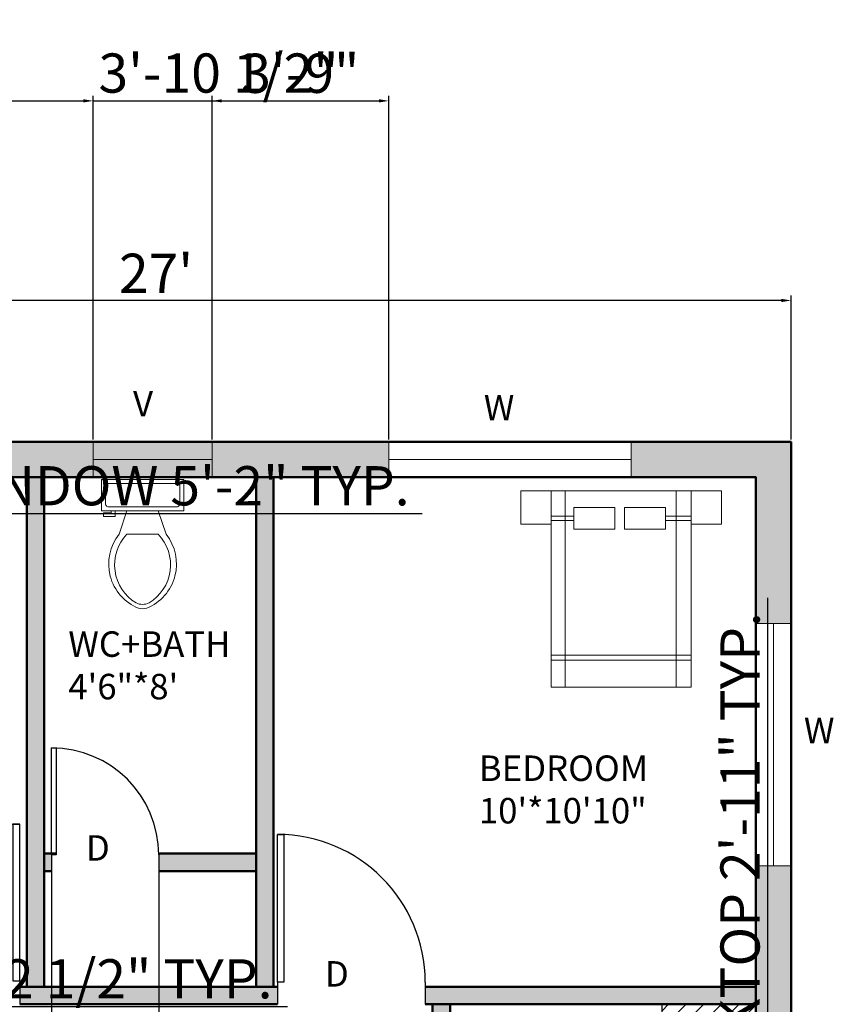
# Model space of a CAD drawing. Units: inches. Extents: x 1935 to 2445, y 1978 to 2806.
# Tile 4 of 4: x 2137 to 2346, y 2554 to 2806. Entities that reach past the tile are written whole.
import ezdxf

# ---------------------------------------------------------------- set-up
doc = ezdxf.new("R2010")
doc.units = ezdxf.units.IN
for name, color, linetype, lineweight in [('A-ANNO-DIMS', 2, 'Continuous', 18), ('A-ANNO-TEXT', 7, 'Continuous', 25), ('A-AREA-IDEN', 130, 'Continuous', 25), ('A-DOOR', 3, 'Continuous', 25), ('A-FLOR-CASE', 123, 'Continuous', 25), ('A-FLOR-CASE-PATT', 123, 'Continuous', 13), ('A-FLOR-FIXT', 9, 'Continuous', 18), ('A-FURN', 9, 'Continuous', 18), ('A-GLAZ', 4, 'Continuous', 18), ('A-WALL-PATT', 225, 'Continuous', 13), ('WALL', 225, 'Continuous', 50)]:
    doc.layers.add(name, color=color, linetype=linetype, lineweight=lineweight)
doc.styles.get("Standard").update_dxf_attribs({"font": 'arial.ttf'})
doc.dimstyles.new('ISO-25', dxfattribs={"dimtxt": 10, "dimasz": 2.5, "dimexe": 1.25, "dimexo": 0.625, "dimtad": 1, "dimdec": 0, "dimlunit": 4, "dimtxsty": 'Standard', "dimcen": 2.5, "dimadec": 0, "dimazin": 0, "dimtfac": 1, "dimtdec": 0, "dimtmove": 0, "dimatfit": 3, "dimfxl": 1, "dimarcsym": 0})

# ---------------------------------------------------------------- blocks, each defined once
blk = doc.blocks.new('*U4')
for p, q in [((9.5, -6), (9.5, -2)), ((-10, -8.5), (-8, -8.5)), ((-10, -9.5), (-10, -8.5)), ((-7, -9.5), (-10, -9.5)), ((-8, -8.5), (-8, -8)), ((-7, -8), (-7, -9.5)), ((-4, -8), (-6, -14)), ((4, -8), (6, -14)), ((4, -14), (-4, -14))]:
    blk.add_line(p, q)
blk.add_lwpolyline([(10.5, -8), (10.5, 0), (-10.5, 0), (-10.5, -8)], close=True)
for points in [[(-9.5, -2), (-9.5, -6)], [(8.5, -1), (-8.5, -1)], [(-8.5, -7), (8.5, -7)]]:
    blk.add_lwpolyline(points)
for centre, radius, start, end in [((-8.62, -1.88), 0.884, 81.8699, 188.1301), ((8.62, -1.88), 0.884, 351.8699, 98.1301), ((-8.62, -6.12), 0.884, 171.8699, 278.1301), ((8.62, -6.12), 0.884, 261.8699, 8.1301), ((3.52, -21.58), 12.17, 141.4691, 247.9714), ((4.2, -21.82), 11.33, 136.3677, 238.9468), ((-3.52, -21.58), 12.17, 292.0284, 38.5307), ((-4.2, -21.82), 11.33, 301.053, 43.6321), ((0, -27.88), 4, 245.7318, 294.2682), ((0, -29), 4, 254.8605, 285.1395)]:
    blk.add_arc(centre, radius, start, end)
blk = doc.blocks.new('*U2')
for p, q in [((0, 0), (0, -6)), ((40, 0), (40, -6))]:
    blk.add_line(p, q)
blk.add_lwpolyline([(0, 0), (0, 40), (1.75, 40), (1.75, 0)], close=True)
blk.add_arc((0, 0), 40, 0, 90)
blk = doc.blocks.new('*D8')
at = {"layer": 'A-ANNO-DIMS', "color": 0, "lineweight": -2, "transparency": 16777216}
for p, q in [((2010.18, 2698.51), (2010.18, 2735.24)), ((2331.68, 2733.99), (2012.68, 2733.99)), ((2334.18, 2698.51), (2334.18, 2735.24))]:
    blk.add_line(p, q, dxfattribs=at)
at = {"layer": 'A-ANNO-DIMS', "color": 0, "lineweight": 100, "transparency": 16777216}
for points in [[(2012.68, 2734.4), (2012.68, 2733.57), (2010.18, 2733.99)], [(2331.68, 2734.4), (2331.68, 2733.57), (2334.18, 2733.99)]]:
    blk.add_solid(points, dxfattribs=at)
at = {"layer": 'Defpoints', "color": 0, "lineweight": 100, "transparency": 16777216}
for p in [(2010.18, 2733.99), (2010.18, 2697.88), (2334.18, 2697.88)]:
    blk.add_point(p, dxfattribs=at)
at = {"layer": 'A-ANNO-DIMS', "color": 0, "transparency": 16777216, "insert": (2172.18, 2739.63), "char_height": 10, "attachment_point": 5}
blk.add_mtext("27'", dxfattribs=at)
blk = doc.blocks.new('*D9')
at = {"layer": 'A-ANNO-DIMS', "color": 0, "lineweight": -2, "transparency": 16777216}
for p, q in [((2333.56, 2697.88), (1952.98, 2697.88)), ((1954.23, 2076.38), (1954.23, 2695.38)), ((2333.56, 2073.88), (1952.98, 2073.88))]:
    blk.add_line(p, q, dxfattribs=at)
at = {"layer": 'A-ANNO-DIMS', "color": 0, "lineweight": 100, "transparency": 16777216}
for points in [[(1953.82, 2695.38), (1954.65, 2695.38), (1954.23, 2697.88)], [(1953.82, 2076.38), (1954.65, 2076.38), (1954.23, 2073.88)]]:
    blk.add_solid(points, dxfattribs=at)
at = {"layer": 'Defpoints', "color": 0, "lineweight": 100, "transparency": 16777216}
for p in [(1954.23, 2697.88), (2334.18, 2697.88), (2334.18, 2073.88)]:
    blk.add_point(p, dxfattribs=at)
at = {"layer": 'A-ANNO-DIMS', "color": 0, "transparency": 16777216, "insert": (1948.5, 2385.88), "char_height": 10, "attachment_point": 5, "rotation": 90}
blk.add_mtext("52'", dxfattribs=at)
blk = doc.blocks.new('WINDOW-STD')
blk.add_line((0, 4.5), (61.82, 4.5))
blk.add_lwpolyline([(0, 9), (61.82, 9), (61.82, 0), (0, 0)], close=True)
blk = doc.blocks.new('VENT-BATH')
blk.add_line((0, 4.5), (30.29, 4.5))
blk.add_lwpolyline([(0, 0), (30.29, 0), (30.29, 9), (0, 9)], close=True)
blk = doc.blocks.new('BED-WITH-NIGHTSTANDS')
for p, q in [((11.32, 50.11), (11.32, 0)), ((39.64, 0), (39.64, 50.11)), ((13.46, 43.65), (7.73, 43.65)), ((43.47, 43.65), (36.85, 43.65)), ((13.46, 42.6), (7.73, 42.6)), ((43.47, 42.6), (36.85, 42.6)), ((7.73, 8.18), (43.47, 8.18)), ((7.73, 6.93), (43.47, 6.93)), ((43.47, 0), (39.64, 0))]:
    blk.add_line(p, q)
for points in [[(0, 50.11), (7.73, 50.11), (7.73, 41.64), (0, 41.64)], [(7.73, 50.11), (43.47, 50.11), (43.47, 0), (7.73, 0)], [(43.47, 50.11), (51.2, 50.11), (51.2, 41.64), (43.47, 41.64)], [(13.46, 45.91), (23.93, 45.91), (23.93, 40.33), (13.46, 40.33)], [(26.4, 45.91), (36.86, 45.91), (36.86, 40.33), (26.4, 40.33)]]:
    blk.add_lwpolyline(points, close=True)
blk = doc.blocks.new('*D18')
at = {"layer": 'A-ANNO-DIMS', "color": 0, "lineweight": -2, "transparency": 16777216}
for p, q in [((2047.95, 2688.26), (2047.95, 2678.36)), ((2109.77, 2688.26), (2109.77, 2678.36)), ((2050.45, 2679.61), (2107.27, 2679.61)), ((2109.77, 2679.61), (2240.06, 2679.61))]:
    blk.add_line(p, q, dxfattribs=at)
at = {"layer": 'A-ANNO-DIMS', "color": 0, "lineweight": 100, "transparency": 16777216}
for points in [[(2050.45, 2680.03), (2050.45, 2679.19), (2047.95, 2679.61)], [(2107.27, 2680.03), (2107.27, 2679.19), (2109.77, 2679.61)]]:
    blk.add_solid(points, dxfattribs=at)
at = {"layer": 'Defpoints', "color": 0, "lineweight": 100, "transparency": 16777216}
for p in [(2047.95, 2688.88), (2109.77, 2688.88), (2109.77, 2679.61)]:
    blk.add_point(p, dxfattribs=at)
at = {"layer": 'A-ANNO-DIMS', "color": 0, "transparency": 16777216, "insert": (2176.16, 2685.41), "char_height": 10, "attachment_point": 5}
blk.add_mtext('WINDOW 5\'-2" TYP.', dxfattribs=at)
blk = doc.blocks.new('*D26')
at = {"layer": 'A-ANNO-DIMS', "color": 0, "lineweight": -2, "transparency": 16777216}
for p, q in [((2022.21, 2552.24), (2022.21, 2555.04)), ((2024.71, 2553.79), (2034.22, 2553.79)), ((2036.72, 2552.24), (2036.72, 2555.04)), ((2036.72, 2553.79), (2205.72, 2553.79))]:
    blk.add_line(p, q, dxfattribs=at)
at = {"layer": 'A-ANNO-DIMS', "color": 0, "lineweight": 100, "transparency": 16777216}
for points in [[(2024.71, 2554.21), (2024.71, 2553.37), (2022.21, 2553.79)], [(2034.22, 2554.21), (2034.22, 2553.37), (2036.72, 2553.79)]]:
    blk.add_solid(points, dxfattribs=at)
at = {"layer": 'Defpoints', "color": 0, "lineweight": 100, "transparency": 16777216}
for p in [(2036.72, 2553.79), (2022.21, 2551.61), (2036.72, 2551.61)]:
    blk.add_point(p, dxfattribs=at)
at = {"layer": 'A-ANNO-DIMS', "color": 0, "transparency": 16777216, "insert": (2122.47, 2559.59), "char_height": 10, "attachment_point": 5}
blk.add_mtext('END TABLE 1\'-2 1/2" TYP.', dxfattribs=at)
blk = doc.blocks.new('*D32')
at = {"layer": 'A-ANNO-DIMS', "color": 0, "lineweight": -2, "transparency": 16777216}
for p, q in [((2328.24, 2511.98), (2328.24, 2658.07)), ((2323.63, 2511.98), (2329.49, 2511.98)), ((2328.24, 2479.6), (2328.24, 2509.48)), ((2323.63, 2477.1), (2329.49, 2477.1))]:
    blk.add_line(p, q, dxfattribs=at)
at = {"layer": 'A-ANNO-DIMS', "color": 0, "lineweight": 100, "transparency": 16777216}
for points in [[(2327.82, 2509.48), (2328.66, 2509.48), (2328.24, 2511.98)], [(2327.82, 2479.6), (2328.66, 2479.6), (2328.24, 2477.1)]]:
    blk.add_solid(points, dxfattribs=at)
at = {"layer": 'Defpoints', "color": 0, "lineweight": 100, "transparency": 16777216}
for p in [(2323.01, 2511.98), (2328.24, 2511.98), (2323.01, 2477.1)]:
    blk.add_point(p, dxfattribs=at)
at = {"layer": 'A-ANNO-DIMS', "color": 0, "transparency": 16777216, "insert": (2322.44, 2586.27), "char_height": 10, "attachment_point": 5, "rotation": 90}
blk.add_mtext('COOKTOP 2\'-11" TYP.', dxfattribs=at)
blk = doc.blocks.new('*D35')
at = {"layer": 'A-ANNO-DIMS', "color": 0, "lineweight": -2, "transparency": 16777216}
for p, q in [((2109.77, 2698.51), (2109.77, 2786.17)), ((2112.27, 2784.92), (2153.67, 2784.92)), ((2156.17, 2698.51), (2156.17, 2786.17)), ((2156.17, 2784.92), (2217.57, 2784.92))]:
    blk.add_line(p, q, dxfattribs=at)
at = {"layer": 'A-ANNO-DIMS', "color": 0, "lineweight": 100, "transparency": 16777216}
for points in [[(2112.27, 2785.34), (2112.27, 2784.51), (2109.77, 2784.92)], [(2153.67, 2785.34), (2153.67, 2784.51), (2156.17, 2784.92)]]:
    blk.add_solid(points, dxfattribs=at)
at = {"layer": 'Defpoints', "color": 0, "lineweight": 100, "transparency": 16777216}
for p in [(2156.17, 2784.92), (2109.77, 2697.88), (2156.17, 2697.88)]:
    blk.add_point(p, dxfattribs=at)
at = {"layer": 'A-ANNO-DIMS', "color": 0, "transparency": 16777216, "insert": (2188.12, 2790.72), "char_height": 10, "attachment_point": 5}
blk.add_mtext('3\'-10 1/2"', dxfattribs=at)
blk = doc.blocks.new('*D36')
at = {"layer": 'A-ANNO-DIMS', "color": 0, "lineweight": -2, "transparency": 16777216}
for p, q in [((2186.46, 2698.51), (2186.46, 2786.17)), ((2188.96, 2784.92), (2229.03, 2784.92)), ((2231.53, 2698.51), (2231.53, 2786.17))]:
    blk.add_line(p, q, dxfattribs=at)
at = {"layer": 'A-ANNO-DIMS', "color": 0, "lineweight": 100, "transparency": 16777216}
for points in [[(2188.96, 2785.34), (2188.96, 2784.51), (2186.46, 2784.92)], [(2229.03, 2785.34), (2229.03, 2784.51), (2231.53, 2784.92)]]:
    blk.add_solid(points, dxfattribs=at)
at = {"layer": 'Defpoints', "color": 0, "lineweight": 100, "transparency": 16777216}
for p in [(2231.53, 2784.92), (2186.46, 2697.88), (2231.53, 2697.88)]:
    blk.add_point(p, dxfattribs=at)
at = {"layer": 'A-ANNO-DIMS', "color": 0, "transparency": 16777216, "insert": (2208.99, 2790.66), "char_height": 10, "attachment_point": 5}
blk.add_mtext('3\'-9"', dxfattribs=at)
blk = doc.blocks.new('*D42')
at = {"layer": 'A-ANNO-DIMS', "color": 0, "lineweight": -2, "transparency": 16777216}
for p, q in [((2145.55, 2591.86), (2145.55, 1986.08)), ((2172.86, 2592.26), (2172.86, 1986.08)), ((2148.05, 1987.33), (2170.36, 1987.33)), ((2172.86, 1987.33), (2226.66, 1987.33))]:
    blk.add_line(p, q, dxfattribs=at)
at = {"layer": 'A-ANNO-DIMS', "color": 0, "lineweight": 100, "transparency": 16777216}
for points in [[(2148.05, 1987.74), (2148.05, 1986.91), (2145.55, 1987.33)], [(2170.36, 1987.74), (2170.36, 1986.91), (2172.86, 1987.33)]]:
    blk.add_solid(points, dxfattribs=at)
at = {"layer": 'Defpoints', "color": 0, "lineweight": 100, "transparency": 16777216}
for p in [(2145.55, 2592.49), (2172.86, 2592.88), (2172.86, 1987.33)]:
    blk.add_point(p, dxfattribs=at)
at = {"layer": 'A-ANNO-DIMS', "color": 0, "transparency": 16777216, "insert": (2201.01, 1993.13), "char_height": 10, "attachment_point": 5}
blk.add_mtext('2\'-3 1/2"', dxfattribs=at)

msp = doc.modelspace()

# ---------------------------------------------------------------- hatches: boundary and pattern name
at = {"layer": 'A-FLOR-CASE-PATT'}
h = msp.add_hatch(dxfattribs=at)
h.set_pattern_fill('ANSI31', color=256)
h.paths.add_polyline_path([(2325.18, 2339.38), (2286.18, 2339.38), (2247.18, 2339.38), (2247.18, 2315.38), (2301.18, 2315.38), (2301.18, 2213.38), (2325.18, 2213.38)])
h.paths.add_polyline_path([(2284.48, 2318.31), (2252.19, 2318.31), (2252.19, 2336.21), (2284.48, 2336.21)], flags=16)
h.paths.add_polyline_path([(2303.5, 2299.32), (2323.01, 2299.32), (2323.01, 2264.44), (2303.5, 2264.44)], flags=16)
h.paths.add_polyline_path([(2317.96, 2291.66, -1), (2307.51, 2291.66, -1)], flags=0)
h.paths.add_polyline_path([(2267.33, 2320), (2253.26, 2320), (2253.26, 2335.01), (2267.33, 2335.01)], flags=0)
h.paths.add_polyline_path([(2258.78, 2327.5, -1), (2261.46, 2327.5, -1)], flags=0)
h.paths.add_polyline_path([(2317.96, 2273.05, -1), (2307.51, 2273.05, -1)], flags=0)
h.paths.add_polyline_path([(2325.18, 2554.38), (2301.18, 2554.38), (2301.18, 2452.38), (2247.18, 2452.38), (2247.18, 2428.38), (2325.18, 2428.38)])
h.paths.add_polyline_path([(2323.01, 2511.98), (2323.01, 2477.1), (2303.5, 2477.1), (2303.5, 2511.98)], flags=16)
h.paths.add_polyline_path([(2317.96, 2504.31, -1), (2307.51, 2504.31, -1)], flags=0)
h.paths.add_polyline_path([(2317.96, 2485.7, -1), (2307.51, 2485.7, -1)], flags=0)
h.paths.add_polyline_path([(2284.48, 2450.03), (2284.48, 2432.13), (2252.19, 2432.13), (2252.19, 2450.03)], flags=16)
h.paths.add_polyline_path([(2267.33, 2448.82), (2267.33, 2433.82), (2253.26, 2433.82), (2253.26, 2448.82)], flags=0)
h.paths.add_polyline_path([(2261.46, 2441.32, -1), (2258.78, 2441.32, -1)], flags=0)
at = {"layer": 'A-WALL-PATT'}
h = msp.add_hatch(color=256, dxfattribs=at)
h.dxf.hatch_style = 1
h.paths.add_polyline_path([(2047.95, 2697.88), (2010.18, 2697.88), (2010.18, 2654.96), (2019.18, 2654.96), (2019.18, 2688.88), (2047.95, 2688.88)], flags=16)
h.paths.add_polyline_path([(2156.17, 2697.88), (2109.77, 2697.88), (2109.77, 2688.88), (2139.18, 2688.88), (2156.17, 2688.88)], flags=17)
h.paths.add_polyline_path([(2231.53, 2697.88), (2186.46, 2697.88), (2186.46, 2688.88), (2231.53, 2688.88)], flags=17)
h.paths.add_polyline_path([(2334.18, 2697.88), (2293.35, 2697.88), (2293.35, 2688.88), (2325.18, 2688.88), (2325.18, 2651.52), (2334.18, 2651.52)], flags=17)
h.paths.add_polyline_path([(2247.18, 2554.38), (2242.68, 2554.38), (2242.68, 2550.71), (2247.18, 2550.71)], flags=17)
h.paths.add_polyline_path([(2145.55, 2592.49), (2145.55, 2592.88), (2143.68, 2592.88), (2143.68, 2588.39), (2145.55, 2588.39)], flags=17)
h.paths.add_polyline_path([(2197.68, 2592.88), (2172.86, 2592.88, -0.003651), (2172.86, 2592.49), (2172.86, 2588.39), (2197.68, 2588.39)], flags=17)
h.paths.add_polyline_path([(2203.16, 2558.88), (2137.4, 2558.88), (2137.4, 2554.38), (2143.68, 2554.38), (2203.16, 2554.38)], flags=17)
h.paths.add_polyline_path([(2097.4, 2558.88), (2019.18, 2558.88), (2019.18, 2554.38), (2097.4, 2554.38)], flags=17)
h.paths.add_polyline_path([(2143.68, 2688.88), (2139.18, 2688.88), (2139.18, 2558.88), (2143.68, 2558.88)], flags=17)
h.paths.add_polyline_path([(2202.18, 2688.88), (2197.68, 2688.88), (2197.68, 2592.88), (2197.68, 2588.39), (2197.68, 2558.88), (2202.18, 2558.88), (2202.18, 2588.38)], flags=17)
h.paths.add_polyline_path([(2241.74, 2229.79), (2251.55, 2229.79), (2251.55, 2243.19), (2241.74, 2243.19)], flags=25)
h.paths.add_polyline_path([(2215.53, 2200.14), (2225.34, 2200.14), (2225.34, 2213.54), (2215.53, 2213.54)], flags=25)
h.paths.add_polyline_path([(2152.61, 2173.98), (2162.42, 2173.98), (2162.42, 2187.38), (2152.61, 2187.38)], flags=25)
h.paths.add_polyline_path([(2109.99, 2200.78), (2119.8, 2200.78), (2119.8, 2214.18), (2109.99, 2214.18)], flags=25)
h.paths.add_polyline_path([(2139.65, 2343.23), (2149.46, 2343.23), (2149.46, 2356.63), (2139.65, 2356.63)], flags=25)
h.paths.add_polyline_path([(2138.05, 2412.22), (2147.87, 2412.22), (2147.87, 2425.62), (2138.05, 2425.62)], flags=25)
h.paths.add_polyline_path([(2242.1, 2526.57), (2251.91, 2526.57), (2251.91, 2539.97), (2242.1, 2539.97)], flags=25)
h.paths.add_polyline_path([(2212.92, 2555.35), (2222.74, 2555.35), (2222.74, 2568.75), (2212.92, 2568.75)], flags=25)
h.paths.add_polyline_path([(2111.94, 2553.1), (2121.75, 2553.1), (2121.75, 2566.5), (2111.94, 2566.5)], flags=25)
h.paths.add_polyline_path([(2032.85, 2161.17), (2083.36, 2161.17), (2083.36, 2185.43), (2032.85, 2185.43)], flags=25)
h.paths.add_polyline_path([(2145.49, 2119.25), (2193.41, 2119.25), (2193.41, 2143.52), (2145.49, 2143.52)], flags=25)
h.paths.add_polyline_path([(2250.93, 2163.1), (2301.44, 2163.1), (2301.44, 2187.36), (2250.93, 2187.36)], flags=25)
h.paths.add_polyline_path([(2247.75, 2274.43), (2290.88, 2274.43), (2290.88, 2298.69), (2247.75, 2298.69)], flags=25)
h.paths.add_polyline_path([(2131.26, 2265.2), (2178.71, 2265.2), (2178.71, 2289.46), (2131.26, 2289.46)], flags=25)
h.paths.add_polyline_path([(2092.71, 2400.61), (2092.71, 2376.16), (2106.11, 2376.16), (2106.11, 2400.61)], flags=25)
h.paths.add_polyline_path([(2173.61, 2396.23), (2189.48, 2396.23), (2189.48, 2409.63), (2173.61, 2409.63)], flags=25)
h.paths.add_polyline_path([(2028.85, 2376.01), (2076.42, 2376.01), (2076.42, 2400.28), (2028.85, 2400.28)], flags=25)
h.paths.add_polyline_path([(2135.3, 2481.1), (2182.75, 2481.1), (2182.75, 2505.37), (2135.3, 2505.37)], flags=25)
h.paths.add_polyline_path([(2249.01, 2476.21), (2292.13, 2476.21), (2292.13, 2500.47), (2249.01, 2500.47)], flags=25)
h.paths.add_polyline_path([(2251.9, 2596.84), (2302.42, 2596.84), (2302.42, 2621.11), (2251.9, 2621.11)], flags=25)
h.paths.add_polyline_path([(2030.66, 2589.83), (2081.18, 2589.83), (2081.18, 2614.09), (2030.66, 2614.09)], flags=25)
h.paths.add_polyline_path([(2019.18, 2593.14), (2010.18, 2593.14), (2010.18, 2520.31), (2019.18, 2520.31)])
h.paths.add_polyline_path([(2010.18, 2164.99), (2019.18, 2164.99), (2019.18, 2238.56), (2010.18, 2238.56)])
h.paths.add_polyline_path([(2048.33, 2073.88), (2048.33, 2082.88), (2019.18, 2082.88), (2019.18, 2103.18), (2010.18, 2103.18), (2010.18, 2073.88)])
h.paths.add_polyline_path([(2156.55, 2073.88), (2156.55, 2082.88), (2110.15, 2082.88), (2110.15, 2073.88)])
h.paths.add_polyline_path([(2231.91, 2073.88), (2231.91, 2082.88), (2186.84, 2082.88), (2186.84, 2073.88)])
h.paths.add_polyline_path([(2047.95, 2688.88), (2047.95, 2697.88), (2010.18, 2697.88), (2010.18, 2654.96), (2019.18, 2654.96), (2019.18, 2688.88)])
h.paths.add_polyline_path([(2109.77, 2697.88), (2109.77, 2688.88), (2156.17, 2688.88), (2156.17, 2697.88)])
h = msp.add_hatch(color=256, dxfattribs=at)
h.dxf.hatch_style = 1
h.paths.add_polyline_path([(2196.68, 2183.38), (2171.78, 2183.38), (2171.78, 2179.29, -0.003687), (2171.78, 2178.88), (2196.68, 2178.88)], flags=17)
h.paths.add_polyline_path([(2144.47, 2183.38), (2142.68, 2183.38), (2142.68, 2178.88), (2144.47, 2178.88), (2144.47, 2179.29)], flags=17)
h.paths.add_polyline_path([(2096.62, 2213.38), (2019.18, 2213.38), (2019.18, 2208.88), (2096.62, 2208.88)], flags=17)
h.paths.add_polyline_path([(2142.68, 2208.88), (2142.68, 2213.38), (2136.62, 2213.38), (2136.62, 2208.88), (2138.18, 2208.88), (2138.18, 2183.38), (2138.18, 2082.88), (2142.68, 2082.88), (2142.68, 2178.88), (2142.68, 2183.38)], flags=17)
h.paths.add_polyline_path([(2201.18, 2208.88), (2202.06, 2208.88), (2202.06, 2213.38), (2196.68, 2213.38), (2196.68, 2204.97), (2196.68, 2082.88), (2201.18, 2082.88)], flags=17)
h.paths.add_polyline_path([(2247.18, 2217.21), (2242.68, 2217.21), (2242.68, 2213.38), (2247.18, 2213.38)], flags=17)
h.paths.add_polyline_path([(2325.18, 2213.38), (2242.68, 2213.38), (2242.68, 2208.88), (2325.18, 2208.88)], flags=17)
h.paths.add_polyline_path([(2247.18, 2339.38), (2242.68, 2339.38), (2242.68, 2257.21), (2247.18, 2257.21)], flags=17)
h.paths.add_polyline_path([(2325.18, 2343.88), (2286.18, 2343.88), (2186.18, 2343.88), (2164.69, 2343.88), (2164.69, 2340.61), (2164.69, 2339.38), (2213.9, 2339.38), (2286.18, 2339.38), (2325.18, 2339.38)], flags=17)
h.paths.add_polyline_path([(2109.68, 2343.88), (2105.18, 2343.88), (2019.18, 2343.88), (2019.18, 2339.38), (2109.68, 2339.38)], flags=17)
h.paths.add_polyline_path([(2120.97, 2340.61), (2120.97, 2343.88), (2109.68, 2343.88), (2109.68, 2339.38), (2120.97, 2339.38)], flags=17)
h.paths.add_polyline_path([(2109.68, 2356.84), (2105.18, 2356.84), (2105.18, 2343.88), (2109.68, 2343.88)], flags=17)
h.paths.add_polyline_path([(2230.51, 2409.48), (2245.95, 2409.48), (2245.95, 2430.09), (2230.51, 2430.09)], flags=25)
h.paths.add_polyline_path([(2289.31, 2409.69), (2322.13, 2409.69), (2322.13, 2430.3), (2289.31, 2430.3)], flags=25)
h.paths.add_polyline_path([(2241.74, 2229.79), (2251.55, 2229.79), (2251.55, 2243.19), (2241.74, 2243.19)], flags=25)
h.paths.add_polyline_path([(2215.53, 2200.14), (2225.34, 2200.14), (2225.34, 2213.54), (2215.53, 2213.54)], flags=25)
h.paths.add_polyline_path([(2152.61, 2173.98), (2162.42, 2173.98), (2162.42, 2187.38), (2152.61, 2187.38)], flags=25)
h.paths.add_polyline_path([(2109.99, 2200.78), (2119.8, 2200.78), (2119.8, 2214.18), (2109.99, 2214.18)], flags=25)
h.paths.add_polyline_path([(2139.65, 2343.23), (2149.46, 2343.23), (2149.46, 2356.63), (2139.65, 2356.63)], flags=25)
h.paths.add_polyline_path([(2138.05, 2412.22), (2147.87, 2412.22), (2147.87, 2425.62), (2138.05, 2425.62)], flags=25)
h.paths.add_polyline_path([(2242.1, 2526.57), (2251.91, 2526.57), (2251.91, 2539.97), (2242.1, 2539.97)], flags=25)
h.paths.add_polyline_path([(2212.92, 2555.35), (2222.74, 2555.35), (2222.74, 2568.75), (2212.92, 2568.75)], flags=25)
h.paths.add_polyline_path([(2151.96, 2587.49), (2161.77, 2587.49), (2161.77, 2600.89), (2151.96, 2600.89)], flags=25)
h.paths.add_polyline_path([(2111.94, 2553.1), (2121.75, 2553.1), (2121.75, 2566.5), (2111.94, 2566.5)], flags=25)
h.paths.add_polyline_path([(2032.85, 2161.17), (2083.36, 2161.17), (2083.36, 2185.43), (2032.85, 2185.43)], flags=25)
h.paths.add_polyline_path([(2145.49, 2119.25), (2193.41, 2119.25), (2193.41, 2143.52), (2145.49, 2143.52)], flags=25)
h.paths.add_polyline_path([(2250.93, 2163.1), (2301.44, 2163.1), (2301.44, 2187.36), (2250.93, 2187.36)], flags=25)
h.paths.add_polyline_path([(2247.75, 2274.43), (2290.88, 2274.43), (2290.88, 2298.69), (2247.75, 2298.69)], flags=25)
h.paths.add_polyline_path([(2131.26, 2265.2), (2178.71, 2265.2), (2178.71, 2289.46), (2131.26, 2289.46)], flags=25)
h.paths.add_polyline_path([(2173.61, 2396.23), (2189.48, 2396.23), (2189.48, 2409.63), (2173.61, 2409.63)], flags=25)
h.paths.add_polyline_path([(2135.3, 2481.1), (2182.75, 2481.1), (2182.75, 2505.37), (2135.3, 2505.37)], flags=25)
h.paths.add_polyline_path([(2249.01, 2476.21), (2292.13, 2476.21), (2292.13, 2500.47), (2249.01, 2500.47)], flags=25)
h.paths.add_polyline_path([(2251.9, 2596.84), (2302.42, 2596.84), (2302.42, 2621.11), (2251.9, 2621.11)], flags=25)
h.paths.add_polyline_path([(2148.05, 2628.52), (2195.98, 2628.52), (2195.98, 2652.78), (2148.05, 2652.78)], flags=25)
h.paths.add_polyline_path([(2030.66, 2589.83), (2081.18, 2589.83), (2081.18, 2614.09), (2030.66, 2614.09)], flags=25)
h.paths.add_polyline_path([(2325.18, 2414.18), (2334.18, 2414.18), (2334.18, 2455.16), (2325.18, 2455.16)])
h.paths.add_polyline_path([(2325.18, 2305.65), (2334.18, 2305.65), (2334.18, 2352.36), (2325.18, 2352.36)])
h.paths.add_polyline_path([(2325.18, 2163.2), (2334.18, 2163.2), (2334.18, 2243.83), (2325.18, 2243.83)])
h.paths.add_polyline_path([(2293.73, 2082.88), (2293.73, 2073.88), (2334.18, 2073.88), (2334.18, 2101.39), (2325.18, 2101.39), (2325.18, 2082.88)])
h.paths.add_polyline_path([(2334.18, 2589.71), (2325.18, 2589.71), (2325.18, 2516.98), (2334.18, 2516.98)])
h.paths.add_polyline_path([(2293.35, 2697.88), (2293.35, 2688.88), (2325.18, 2688.88), (2325.18, 2651.52), (2334.18, 2651.52), (2334.18, 2697.88)])
h.paths.add_polyline_path([(2109.77, 2697.88), (2109.77, 2688.88), (2231.53, 2688.88), (2231.53, 2697.88)])
h.paths.add_polyline_path([(2010.18, 2654.96), (2019.18, 2654.96), (2019.18, 2688.88), (2047.95, 2688.88), (2047.95, 2697.88), (2010.18, 2697.88)])
h.paths.add_polyline_path([(2010.18, 2520.31), (2019.18, 2520.31), (2019.18, 2593.14), (2010.18, 2593.14)])
h = msp.add_hatch(color=256, dxfattribs=at)
h.dxf.hatch_style = 1
h.paths.add_polyline_path([(2334.18, 2589.71), (2325.18, 2589.71), (2325.18, 2516.98), (2334.18, 2516.98)])
h.paths.add_polyline_path([(2325.18, 2558.88), (2240.84, 2558.88), (2240.84, 2554.38), (2325.18, 2554.38)])
h.paths.add_polyline_path([(2119.73, 2427.16), (2119.73, 2428.38), (2019.18, 2428.38), (2019.18, 2423.88), (2119.73, 2423.88)])
h.paths.add_polyline_path([(2230.51, 2409.48), (2245.95, 2409.48), (2245.95, 2430.09), (2230.51, 2430.09)], flags=9)
h.paths.add_polyline_path([(2289.31, 2409.69), (2322.13, 2409.69), (2322.13, 2430.3), (2289.31, 2430.3)], flags=9)
h.paths.add_polyline_path([(2241.74, 2229.79), (2251.55, 2229.79), (2251.55, 2243.19), (2241.74, 2243.19)], flags=9)
h.paths.add_polyline_path([(2215.53, 2200.14), (2225.34, 2200.14), (2225.34, 2213.54), (2215.53, 2213.54)], flags=9)
h.paths.add_polyline_path([(2152.61, 2173.98), (2162.42, 2173.98), (2162.42, 2187.38), (2152.61, 2187.38)], flags=9)
h.paths.add_polyline_path([(2109.99, 2200.78), (2119.8, 2200.78), (2119.8, 2214.18), (2109.99, 2214.18)], flags=9)
h.paths.add_polyline_path([(2139.65, 2343.23), (2149.46, 2343.23), (2149.46, 2356.63), (2139.65, 2356.63)], flags=9)
h.paths.add_polyline_path([(2138.05, 2412.22), (2147.87, 2412.22), (2147.87, 2425.62), (2138.05, 2425.62)], flags=9)
h.paths.add_polyline_path([(2242.1, 2526.57), (2251.91, 2526.57), (2251.91, 2539.97), (2242.1, 2539.97)], flags=9)
h.paths.add_polyline_path([(2212.92, 2555.35), (2222.74, 2555.35), (2222.74, 2568.75), (2212.92, 2568.75)], flags=9)
h.paths.add_polyline_path([(2151.96, 2587.49), (2161.77, 2587.49), (2161.77, 2600.89), (2151.96, 2600.89)], flags=9)
h.paths.add_polyline_path([(2111.94, 2553.1), (2121.75, 2553.1), (2121.75, 2566.5), (2111.94, 2566.5)], flags=9)
h.paths.add_polyline_path([(2032.85, 2161.17), (2083.36, 2161.17), (2083.36, 2185.43), (2032.85, 2185.43)], flags=9)
h.paths.add_polyline_path([(2145.49, 2119.25), (2193.41, 2119.25), (2193.41, 2143.52), (2145.49, 2143.52)], flags=9)
h.paths.add_polyline_path([(2250.93, 2163.1), (2301.44, 2163.1), (2301.44, 2187.36), (2250.93, 2187.36)], flags=9)
h.paths.add_polyline_path([(2247.75, 2274.43), (2290.88, 2274.43), (2290.88, 2298.69), (2247.75, 2298.69)], flags=9)
h.paths.add_polyline_path([(2131.26, 2265.2), (2178.71, 2265.2), (2178.71, 2289.46), (2131.26, 2289.46)], flags=9)
h.paths.add_polyline_path([(2173.61, 2396.23), (2189.48, 2396.23), (2189.48, 2409.63), (2173.61, 2409.63)], flags=9)
h.paths.add_polyline_path([(2135.3, 2481.1), (2182.75, 2481.1), (2182.75, 2505.37), (2135.3, 2505.37)], flags=9)
h.paths.add_polyline_path([(2249.01, 2476.21), (2292.13, 2476.21), (2292.13, 2500.47), (2249.01, 2500.47)], flags=9)
h.paths.add_polyline_path([(2251.9, 2596.84), (2302.42, 2596.84), (2302.42, 2621.11), (2251.9, 2621.11)], flags=9)
h.paths.add_polyline_path([(2148.05, 2628.52), (2195.98, 2628.52), (2195.98, 2652.78), (2148.05, 2652.78)], flags=9)
h.paths.add_polyline_path([(2030.66, 2589.83), (2081.18, 2589.83), (2081.18, 2614.09), (2030.66, 2614.09)], flags=9)

# ---------------------------------------------------------------- linework, layer by layer
at = {"layer": 'A-FLOR-CASE'}
for p, q in [((2325.18, 2554.38), (2301.18, 2554.38)), ((2301.18, 2554.38), (2301.18, 2452.38))]:
    msp.add_line(p, q, dxfattribs=at)
at = {"layer": 'WALL'}
for p, q in [((2019.18, 2688.88), (2139.18, 2688.88)), ((2139.18, 2688.88), (2139.18, 2558.88)), ((2143.68, 2688.88), (2143.68, 2558.88)), ((2143.68, 2688.88), (2197.68, 2688.88)), ((2197.68, 2688.88), (2197.68, 2592.88)), ((2202.18, 2688.88), (2202.18, 2588.38)), ((2146.74, 2592.88), (2143.68, 2592.88)), ((2197.68, 2592.88), (2172.86, 2592.88)), ((2197.68, 2592.88), (2197.68, 2558.88)), ((2145.55, 2588.39), (2143.68, 2588.39)), ((2143.68, 2588.39), (2145.55, 2588.39)), ((2172.86, 2588.39), (2197.68, 2588.39)), ((2202.18, 2588.38), (2202.18, 2558.88)), ((2139.18, 2558.88), (2137.4, 2558.88)), ((2137.4, 2558.88), (2203.16, 2558.88)), ((2240.84, 2558.88), (2325.18, 2558.88)), ((2143.68, 2554.38), (2137.4, 2554.38)), ((2143.68, 2554.38), (2203.16, 2554.38)), ((2240.84, 2554.38), (2325.18, 2554.38)), ((2242.68, 2550.71), (2242.68, 2554.38)), ((2247.18, 2550.71), (2247.18, 2554.38)), ((2325.18, 2554.38), (2325.18, 2428.38))]:
    msp.add_line(p, q, dxfattribs=at)
for points in [[(2010.18, 2073.88), (2334.18, 2073.88), (2334.18, 2697.88), (2010.18, 2697.88)], [(2019.18, 2082.88), (2325.18, 2082.88), (2325.18, 2688.88), (2019.18, 2688.88)]]:
    msp.add_lwpolyline(points, close=True, dxfattribs=at)

# ---------------------------------------------------------------- block references
at = {"layer": 'A-DOOR'}
for p, xscale, yscale, zscale in [((2145.55, 2592.49), 0.6828645758789585, 0.6828645758789585, 0.6828645758789585), ((2203.16, 2560.04), 0.9420900055362247, 0.9420900055362247, 0.9420900055362247)]:
    msp.add_blockref('*U2', p, dxfattribs=dict(at, xscale=xscale, yscale=yscale, zscale=zscale))
at = {"layer": 'A-DOOR', "xscale": -1}
msp.add_blockref('*U2', (2137.4, 2560.38), dxfattribs=at)
at = {"layer": 'A-FLOR-FIXT'}
msp.add_blockref('*U4', (2168.75, 2688.32), dxfattribs=at)
at = {"layer": 'A-FURN'}
msp.add_blockref('BED-WITH-NIGHTSTANDS', (2265.25, 2635.28), dxfattribs=at)
at = {"layer": 'A-GLAZ'}
for name, p in [('VENT-BATH', (2156.17, 2688.88)), ('WINDOW-STD', (2231.53, 2688.88))]:
    msp.add_blockref(name, p, dxfattribs=at)
at = {"layer": 'A-GLAZ', "rotation": 270.0000000000006}
msp.add_blockref('WINDOW-STD', (2325.18, 2651.52), dxfattribs=at)

# ---------------------------------------------------------------- texts
at = {"layer": 'A-ANNO-TEXT', "char_height": 6.5, "attachment_point": 1}
for s, insert in [('V', (2166.31, 2710.89)), ('W', (2255.79, 2709.88)), ('W', (2337.45, 2627.49)), ('D', (2154.28, 2597.54)), ('D', (2215.25, 2565.4))]:
    msp.add_mtext_dynamic_manual_height_columns(s, width=118.8911, gutter_width=32.51, heights=[0], dxfattribs=dict(at, insert=insert))
at = {"layer": 'A-AREA-IDEN', "char_height": 6.503, "attachment_point": 1}
for s, insert in [('WC+BATH\\P4\'6"*8\'', (2149.8, 2649.55)), ('BEDROOM\\P10\'*10\'10"', (2254.52, 2617.88))]:
    msp.add_mtext_dynamic_manual_height_columns(s, width=118.8911, gutter_width=32.51, heights=[0], dxfattribs=dict(at, insert=insert))

# ---------------------------------------------------------------- dimensions: what is measured, and where the dimension line sits
at = {"layer": 'A-ANNO-DIMS'}
for base, p1, p2, override, picture, middle in [((2156.17, 2784.92), (2109.77, 2697.88), (2156.17, 2697.88), {"dimdec": 1, "dimlfac": 1, "dimrnd": 0, "dimzin": 1, "dimdsep": 46, "dimlunit": 4, "dimfrac": 2}, '*D35', (2188.12, 2790.72)), ((2231.53, 2784.92), (2186.46, 2697.88), (2231.53, 2697.88), {"dimdec": 1, "dimlfac": 1, "dimrnd": 0, "dimzin": 1, "dimdsep": 46, "dimlunit": 4, "dimfrac": 2}, '*D36', (2208.99, 2790.66)), ((2010.18, 2733.99), (2334.18, 2697.88), (2010.18, 2697.88), {"dimclrd": 0, "dimclre": 0, "dimclrt": 0}, '*D8', (2172.18, 2739.63)), ((2172.86, 1987.33), (2145.55, 2592.49), (2172.86, 2592.88), {"dimdec": 1, "dimlfac": 1, "dimrnd": 0, "dimzin": 1, "dimdsep": 46, "dimlunit": 4, "dimfrac": 2}, '*D42', (2201.01, 1993.13))]:
    dim = msp.add_linear_dim(base=base, p1=p1, p2=p2, dimstyle='ISO-25', override=override, dxfattribs=at)
    dim.commit()
    dim.dimension.update_dxf_attribs({"geometry": picture, "text_midpoint": middle})
for base, p1, p2, text, picture, middle in [((2109.77, 2679.61), (2047.95, 2688.88), (2109.77, 2688.88), 'WINDOW <> TYP.', '*D18', (2176.16, 2685.41)), ((2036.72, 2553.79), (2022.21, 2551.61), (2036.72, 2551.61), 'END TABLE <> TYP.', '*D26', (2122.47, 2559.59))]:
    dim = msp.add_linear_dim(base=base, p1=p1, p2=p2, text=text, dimstyle='ISO-25', override={"dimdec": 1, "dimlfac": 1, "dimrnd": 0, "dimzin": 1, "dimdsep": 46, "dimlunit": 4, "dimfrac": 2}, dxfattribs=at)
    dim.commit()
    dim.dimension.update_dxf_attribs({"geometry": picture, "text_midpoint": middle})
dim = msp.add_linear_dim(base=(1954.23, 2697.88), p1=(2334.18, 2073.88), p2=(2334.18, 2697.88), angle=90, dimstyle='ISO-25', override={"dimclrd": 0, "dimclre": 0, "dimclrt": 0}, dxfattribs=at)
dim.commit()
dim.dimension.update_dxf_attribs({"geometry": '*D9', "text_midpoint": (1948.5, 2385.88)})
dim = msp.add_linear_dim(base=(2328.24, 2511.98), p1=(2323.01, 2477.1), p2=(2323.01, 2511.98), angle=90, text='COOKTOP <> TYP.', dimstyle='ISO-25', override={"dimdec": 1, "dimlfac": 1, "dimrnd": 0, "dimzin": 1, "dimdsep": 46, "dimlunit": 4, "dimfrac": 2}, dxfattribs=at)
dim.commit()
dim.dimension.update_dxf_attribs({"geometry": '*D32', "text_midpoint": (2322.44, 2586.27)})

doc.saveas('drawing.dxf')
